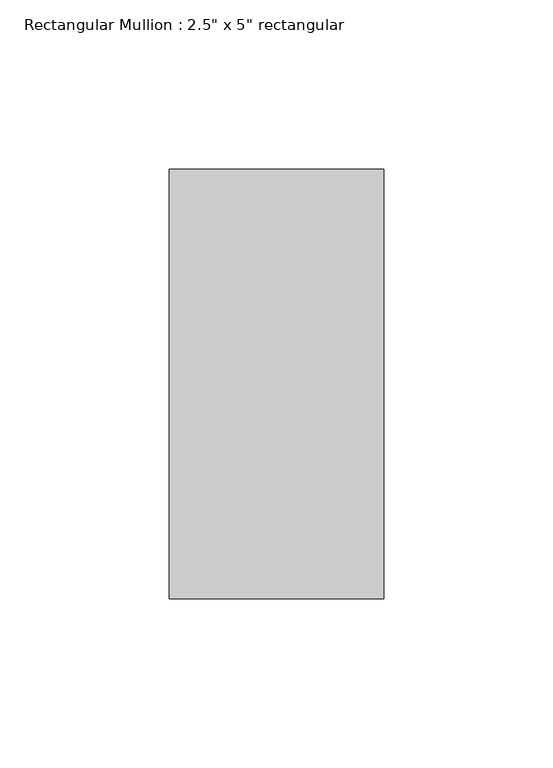
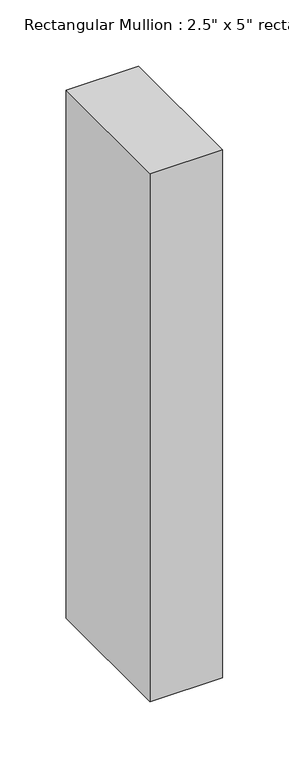
"""IFC4 building model written with IfcOpenShell, lengths in millimetres: member geometry."""

from ifc_helpers import new_model, si_unit, frame, origin, place, context, project, spatial, polyline, outline, extrude, source, transform, mapped, element, save


def member_1d451195(model_context):
    return source(origin(), model_context, "Body", "SweptSolid", [
        extrude(outline(polyline([(0.0, 63.5), (0.0, -63.5), (-63.5, -63.5), (-63.5, 63.5), (0.0, 63.5)])), frame((0.0, 0.0, -487.4598371), z_axis=(0.0, 0.0, 1.0), x_axis=(1.0, 0.0, 0.0)), (0.0, 0.0, 1.0), 487.4598371),
    ])


if __name__ == "__main__":
    model = new_model("IFC4")
    model_context = context("Model", 3, world=origin())
    ifc_project = project(units=[si_unit("LENGTHUNIT", "METRE", prefix="MILLI")], contexts=[model_context])
    site = spatial("IfcSite", under=ifc_project)
    building = spatial("IfcBuilding", under=site)
    placement = place(None, origin())
    member_shape = member_1d451195(model_context)
    element("IfcMember", 1, ObjectType="Rectangular Mullion : 2.5\" x 5\" rectangular", at=placement, inside=building, context=model_context, shape_type="MappedRepresentation", body=[
        mapped(member_shape, transform((0.0, 0.0, 0.0), x_axis=(1.0, 0.0, 0.0), y_axis=(0.0, 1.0, 0.0), z_axis=(0.0, 0.0, 1.0))),
    ])
    save(model, "model.ifc")

# Revit data of these elements
# Type "Rectangular Mullion : 2.5\" x 5\" rectangular"
#   built-in parameter 1007304 = 0.416667 (stored number, unit not read)
#   built-in parameter 1007301 = 0.104167 (stored number, unit not read)
#   built-in parameter 1007300 = 0.104167 (stored number, unit not read)
# Element 1 (IfcMember, "Rectangular Mullion : 2.5\" x 5\" rectangular")
#   Materials on its faces: "mullions"
# Materials
#   "mullions": class "Generic", colour RGB 120 120 120, transparency 0, Cost = 0
